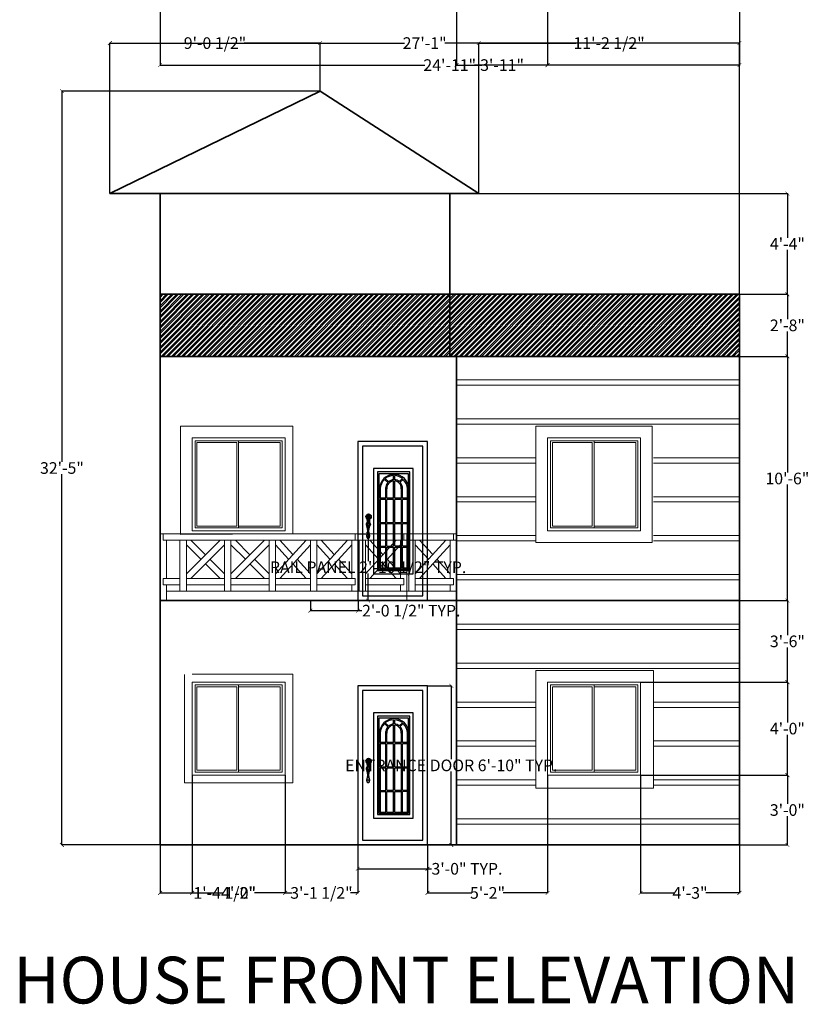
# Model space of a CAD drawing. Units: inches. Extents: x 528 to 2520, y -151 to 1354.
# Tile 28 of 41: x 2086 to 2493, y -151 to 357. Entities that reach past the tile are written whole.
import ezdxf

# ---------------------------------------------------------------- set-up
doc = ezdxf.new("R2010")
doc.units = ezdxf.units.IN
doc.header["$MEASUREMENT"] = 0
for name, color, linetype, lineweight in [('A-ANNO-DIMS', 2, 'Continuous', 18), ('A-ANNO-TEXT', 7, 'Continuous', 30), ('A-Door', 150, 'Continuous', 25), ('A-ELEV', 7, 'Continuous', 35), ('A-ELEV-FNSH', 7, 'Continuous', 18), ('A-ROOF', 7, 'Continuous', 35), ('KORKULUK', 4, 'Continuous', 20), ('WINDOWS', 2, 'Continuous', 20)]:
    doc.layers.add(name, color=color, linetype=linetype, lineweight=lineweight)
doc.layers.add('A-ELEV-PATT', color=175, linetype='Continuous', lineweight=13, true_color=0x4554a5)
doc.styles.get("Standard").update_dxf_attribs({"font": 'arial.ttf'})
doc.dimstyles.get("Standard").update_dxf_attribs({"dimtxt": 6, "dimasz": 2, "dimexe": 0.18, "dimexo": 0.0625, "dimgap": 0.09, "dimtad": 0, "dimtih": 1, "dimtoh": 1, "dimdec": 1, "dimzin": 0, "dimdsep": 46, "dimlunit": 3, "dimtxsty": 'Standard', "dimblk": 'ARCHTICK', "dimcen": 0.09, "dimadec": 0, "dimazin": 0, "dimtfac": 1, "dimtdec": 1, "dimtofl": 0, "dimtmove": 0, "dimatfit": 3, "dimfxl": 1, "dimtolj": 1, "dimtzin": 0, "dimarcsym": 0})

# ---------------------------------------------------------------- blocks, each defined once
blk = doc.blocks.new('*U29')
for p, q in [((1.5, 1.5), (1.5, 46.5)), ((1.5, 46.5), (24, 46.5)), ((24, 1.5), (24, 46.5)), ((24, 46.5), (46.5, 46.5)), ((46.5, 46.5), (46.5, 1.5)), ((24, 1.5), (1.5, 1.5)), ((46.5, 1.5), (24, 1.5))]:
    blk.add_line(p, q)
blk.add_lwpolyline([(0, 0), (0, 48), (48, 48), (48, 0)], close=True)
for points in [[(23, 45.5), (23, 2.5), (2.5, 2.5), (2.5, 45.5), (23, 45.5)], [(24, 45.5), (45.5, 45.5), (45.5, 2.5), (24, 2.5)]]:
    blk.add_lwpolyline(points)
blk = doc.blocks.new('DOOR-PANEL-ELEV-36')
for p, q in [((13.74, 62.55), (15.59, 60.9)), ((14.17, 62.94), (16, 61.3)), ((18.52, 62.33), (18.52, 64.55)), ((18.52, 52.78), (18.52, 61.75)), ((19.1, 62.33), (19.1, 64.53)), ((19.1, 52.78), (19.1, 61.75)), ((23.08, 62.95), (21.41, 61.45)), ((23.52, 62.56), (21.85, 61.06)), ((11.91, 57.81), (11.37, 57.81)), ((11.6, 57.81), (11.83, 57.81)), ((11.91, 57.81), (11.6, 57.81)), ((11.83, 57.81), (11.83, 58.12)), ((14.52, 52.78), (14.52, 58.42)), ((15.1, 52.78), (15.1, 58.42)), ((22.52, 52.78), (22.52, 58.12)), ((23.1, 52.78), (23.1, 58.12)), ((14.52, 52.78), (11.55, 52.78)), ((14.52, 52.2), (11.55, 52.2)), ((14.52, 40.31), (14.52, 52.2)), ((18.52, 52.78), (15.1, 52.78)), ((15.1, 40.31), (15.1, 52.2)), ((18.52, 52.2), (15.1, 52.2)), ((18.52, 40.33), (18.52, 52.2)), ((22.52, 52.78), (19.1, 52.78)), ((19.1, 40.33), (19.1, 52.2)), ((22.52, 52.2), (19.1, 52.2)), ((22.52, 40.35), (22.52, 52.2)), ((25.61, 52.78), (23.1, 52.78)), ((25.61, 52.2), (23.1, 52.2)), ((23.1, 40.36), (23.1, 52.2)), ((5.17, 42.07), (5.17, 40.37)), ((5.85, 42.01), (5.85, 40.4)), ((5.17, 38.33), (5.17, 34.66)), ((5.6, 38.27), (5.6, 34.75)), ((11.55, 40.29), (14.52, 40.31)), ((11.55, 39.71), (14.52, 39.73)), ((14.52, 28.17), (14.52, 39.73)), ((15.1, 40.31), (18.52, 40.33)), ((15.1, 39.73), (18.52, 39.75)), ((15.1, 28.17), (15.1, 39.73)), ((18.52, 28.19), (18.52, 39.75)), ((19.1, 40.33), (22.52, 40.35)), ((19.1, 39.76), (22.52, 39.78)), ((19.1, 28.19), (19.1, 39.76)), ((22.52, 16.87), (22.52, 39.78)), ((23.1, 40.36), (25.61, 40.37)), ((23.1, 39.78), (25.61, 39.8)), ((23.1, 28.22), (23.1, 39.78)), ((10.97, 16.3), (10.97, 27.86)), ((11.55, 28.15), (14.52, 28.17)), ((11.55, 27.57), (14.52, 27.59)), ((14.52, 16.87), (14.52, 27.59)), ((15.1, 28.17), (18.52, 28.19)), ((15.1, 27.59), (18.52, 27.61)), ((15.1, 16.87), (15.1, 27.59)), ((18.52, 16.87), (18.52, 27.61)), ((19.1, 28.19), (22.52, 28.21)), ((19.1, 27.62), (22.52, 27.64)), ((19.1, 16.87), (19.1, 27.62)), ((23.1, 28.22), (25.61, 28.23)), ((23.1, 27.64), (25.61, 27.66)), ((23.1, 16.87), (23.1, 27.64)), ((26.23, 16.3), (22.52, 16.3))]:
    blk.add_line(p, q)
for points in [[(36, 0), (36, 82.04), (0, 82.04), (0, 0)], [(33.55, 2.45), (33.55, 79.6), (2.45, 79.6), (2.45, 2.45)], [(28.61, 13.88), (28.61, 68.17), (8.2, 68.17), (8.2, 13.88)], [(26.88, 15.61), (26.88, 66.44), (10.28, 66.44), (10.28, 15.61)], [(26.19, 16.3), (26.19, 65.4), (10.97, 65.4), (10.97, 16.3)], [(6.31, 42.2), (6.31, 44.42), (4.84, 44.42), (4.84, 42.2)], [(5.86, 42.6), (5.86, 43.89), (5.29, 43.89), (5.29, 42.6)], [(6, 38.52), (6, 40.2), (4.97, 40.2), (4.97, 38.52)]]:
    blk.add_lwpolyline(points, close=True)
for points in [[(11.55, 58.12), (11.55, 52.78)], [(25.61, 52.78), (25.61, 59.08)], [(11.55, 52.2), (11.55, 40.29)], [(25.61, 40.37), (25.61, 52.2)], [(11.55, 39.71), (11.55, 16.87), (14.52, 16.87)], [(25.61, 16.87), (25.61, 39.8)], [(15.1, 16.87), (18.52, 16.87)], [(19.1, 16.87), (22.52, 16.87)], [(23.1, 16.87), (25.61, 16.87)]]:
    blk.add_lwpolyline(points)
blk.add_lwpolyline([(6.03, 33.36, -0.045721), (5.98, 32.78, -0.059301), (5.85, 32.36, -0.101058), (5.61, 32.02, -0.189275), (5.4, 31.94, -0.189275), (5.19, 32.02, -0.101058), (4.95, 32.36, -0.059301), (4.82, 32.78, -0.045721), (4.77, 33.36, -0.045721), (4.82, 33.94, -0.059301), (4.95, 34.37, -0.101058), (5.19, 34.7, -0.189275), (5.4, 34.78, -0.189275), (5.61, 34.7, -0.101058), (5.85, 34.37, -0.059301), (5.98, 33.94, -0.045721)], format="xyb", close=True)
for centre, radius in [((5.61, 43.34), 1.35), ((5.61, 43.34), 0.752), ((5.61, 43.34), 0.392), ((5.5, 39.36), 1.05), ((5.5, 39.36), 0.55), ((5.39, 33.33), 0.278)]:
    blk.add_circle(centre, radius)
for centre, radius, start, end in [((18.79, 57.56), 7.57, 1.2104, 178.7896), ((18.64, 57.56), 6.99, 134.4827, 178.7896), ((18.64, 57.56), 6.99, 90.9488, 129.7225), ((18.79, 58.05), 3.71, 94.2253, 185.0935), ((18.79, 58.05), 4.29, 93.6561, 130.6705), ((19.88, 38.4), 27.02, 89.5366, 91.7216), ((18.64, 57.56), 6.99, 50.4895, 86.2145), ((18.79, 58.05), 4.29, 52.4124, 85.9434), ((18.79, 58.05), 3.71, 354.9065, 85.3116), ((18.79, 58.05), 4.29, 354.9065, 44.6486), ((18.64, 57.56), 6.99, 1.2104, 45.7292), ((18.79, 58.05), 4.29, 138.3994, 185.0935), ((2.68, 41.16), 2.34, 319.4574, 32.1732), ((8.36, 40.89), 2.34, 142.3675, 215.0833), ((-1.32, 36.06), 6.5, 338.0978, 21.9022), ((12.13, 36.06), 6.5, 158.0978, 201.9022)]:
    blk.add_arc(centre, radius, start, end)
blk = doc.blocks.new('BALCONY-RAIL-PANEL')
for p, q in [((0, 31.17), (0, 4.92)), ((3.28, 31.17), (3.28, 4.92)), ((3.28, 13.91), (19.11, 31.17)), ((5.51, 31.17), (12.31, 23.75)), ((21.34, 31.17), (21.34, 11.48)), ((24.62, 34.45), (24.62, 0)), ((3.28, 28.74), (10.08, 21.33)), ((5.51, 11.48), (21.34, 28.74)), ((14.54, 21.33), (21.34, 13.91)), ((12.31, 18.9), (19.11, 11.48)), ((3.28, 11.48), (23.05, 11.48)), ((3.28, 8.2), (23.05, 8.2)), ((21.34, 8.2), (21.34, 4.92))]:
    blk.add_line(p, q)
for points in [[(23.05, 31.17), (23.05, 34.45)], [(23.05, 8.2), (23.05, 11.48)]]:
    blk.add_lwpolyline(points)
blk = doc.blocks.new('_ArchTick')
at = {"color": 0, "linetype": 'ByBlock', "const_width": 0.15}
blk.add_lwpolyline([(-0.5, -0.5), (0.5, 0.5)], dxfattribs=at)
blk = doc.blocks.new('*D88')
at = {"layer": 'A-ANNO-DIMS', "color": 0, "lineweight": -2, "transparency": 16777216}
for p, q in [((2260.28, 91.5), (2265.56, 91.5)), ((2265.38, 91.5), (2265.38, 77.47)), ((2265.38, 57.05), (2265.38, 71.08)), ((2260.28, 57.05), (2265.56, 57.05))]:
    blk.add_line(p, q, dxfattribs=at)
at = {"layer": 'Defpoints', "color": 0, "transparency": 16777216}
for p in [(2260.22, 91.5), (2265.38, 91.5), (2260.22, 57.05)]:
    blk.add_point(p, dxfattribs=at)
at = {"layer": 'A-ANNO-DIMS', "color": 0, "lineweight": -2, "transparency": 16777216, "xscale": 2, "yscale": 2, "zscale": 2}
for p, rotation in [((2265.38, 91.5), 90), ((2265.38, 57.05), 270)]:
    blk.add_blockref('_ArchTick', p, dxfattribs=dict(at, rotation=rotation))
at = {"layer": 'A-ANNO-DIMS', "color": 0, "transparency": 16777216, "insert": (2265.38, 74.27), "char_height": 6, "attachment_point": 5}
blk.add_mtext('\\A1;RAIL PANEL 2\'-10 1/2" TYP.', dxfattribs=at)
blk = doc.blocks.new('*D89')
at = {"layer": 'A-ANNO-DIMS', "color": 0, "lineweight": -2, "transparency": 16777216}
for p, q in [((2235.6, 56.99), (2235.6, 51.7)), ((2260.22, 56.99), (2260.22, 51.7)), ((2235.6, 51.88), (2260.22, 51.88)), ((2260.22, 51.88), (2262.22, 51.88))]:
    blk.add_line(p, q, dxfattribs=at)
at = {"layer": 'Defpoints', "color": 0, "transparency": 16777216}
for p in [(2235.6, 57.05), (2260.22, 57.05), (2260.22, 51.88)]:
    blk.add_point(p, dxfattribs=at)
at = {"layer": 'A-ANNO-DIMS', "color": 0, "lineweight": -2, "transparency": 16777216, "xscale": 2, "yscale": 2, "zscale": 2, "rotation": 180}
blk.add_blockref('_ArchTick', (2235.6, 51.88), dxfattribs=at)
at = {"layer": 'A-ANNO-DIMS', "color": 0, "lineweight": -2, "transparency": 16777216, "xscale": 2, "yscale": 2, "zscale": 2}
blk.add_blockref('_ArchTick', (2260.22, 51.88), dxfattribs=at)
at = {"layer": 'A-ANNO-DIMS', "color": 0, "transparency": 16777216, "insert": (2287.64, 51.88), "char_height": 6, "attachment_point": 5}
blk.add_mtext('\\A1;2\'-0 1/2" TYP.', dxfattribs=at)
blk = doc.blocks.new('*D90')
at = {"layer": 'A-ANNO-DIMS', "color": 0, "lineweight": -2, "transparency": 16777216}
for p, q in [((2296.08, 13.09), (2308.5, 13.09)), ((2308.32, 13.09), (2308.32, -24.73)), ((2308.32, -68.95), (2308.32, -31.12)), ((2296.08, -68.95), (2308.5, -68.95))]:
    blk.add_line(p, q, dxfattribs=at)
at = {"layer": 'Defpoints', "color": 0, "transparency": 16777216}
for p in [(2296.02, 13.09), (2308.32, 13.09), (2296.02, -68.95)]:
    blk.add_point(p, dxfattribs=at)
at = {"layer": 'A-ANNO-DIMS', "color": 0, "lineweight": -2, "transparency": 16777216, "xscale": 2, "yscale": 2, "zscale": 2}
for p, rotation in [((2308.32, 13.09), 90), ((2308.32, -68.95), 270)]:
    blk.add_blockref('_ArchTick', p, dxfattribs=dict(at, rotation=rotation))
at = {"layer": 'A-ANNO-DIMS', "color": 0, "transparency": 16777216, "insert": (2308.32, -27.93), "char_height": 6, "attachment_point": 5}
blk.add_mtext('\\A1;ENTRANCE DOOR 6\'-10" TYP.', dxfattribs=at)
blk = doc.blocks.new('*D91')
at = {"layer": 'A-ANNO-DIMS', "color": 0, "lineweight": -2, "transparency": 16777216}
for p, q in [((2260.02, -69.01), (2260.02, -81.44)), ((2296.02, -69.01), (2296.02, -81.44)), ((2260.02, -81.26), (2296.02, -81.26)), ((2296.02, -81.26), (2298.02, -81.26))]:
    blk.add_line(p, q, dxfattribs=at)
at = {"layer": 'Defpoints', "color": 0, "transparency": 16777216}
for p in [(2260.02, -68.95), (2296.02, -68.95), (2296.02, -81.26)]:
    blk.add_point(p, dxfattribs=at)
at = {"layer": 'A-ANNO-DIMS', "color": 0, "lineweight": -2, "transparency": 16777216, "xscale": 2, "yscale": 2, "zscale": 2, "rotation": 180}
blk.add_blockref('_ArchTick', (2260.02, -81.26), dxfattribs=at)
at = {"layer": 'A-ANNO-DIMS', "color": 0, "lineweight": -2, "transparency": 16777216, "xscale": 2, "yscale": 2, "zscale": 2}
blk.add_blockref('_ArchTick', (2296.02, -81.26), dxfattribs=at)
at = {"layer": 'A-ANNO-DIMS', "color": 0, "transparency": 16777216, "insert": (2316.39, -81.26), "char_height": 6, "attachment_point": 5}
blk.add_mtext('\\A1;3\'-0" TYP.', dxfattribs=at)
blk = doc.blocks.new('*D94')
at = {"layer": 'A-ANNO-DIMS', "color": 0, "lineweight": -2, "transparency": 16777216}
for p, q in [((2158.01, 360.88), (2158.01, 333.11)), ((2457.01, 360.88), (2457.01, 333.11)), ((2158.01, 333.29), (2294.73, 333.29)), ((2457.01, 333.29), (2320.29, 333.29))]:
    blk.add_line(p, q, dxfattribs=at)
at = {"layer": 'Defpoints', "color": 0, "transparency": 16777216}
for p in [(2158.01, 360.94), (2457.01, 360.94), (2457.01, 333.29)]:
    blk.add_point(p, dxfattribs=at)
at = {"layer": 'A-ANNO-DIMS', "color": 0, "lineweight": -2, "transparency": 16777216, "xscale": 2, "yscale": 2, "zscale": 2, "rotation": 180}
blk.add_blockref('_ArchTick', (2158.01, 333.29), dxfattribs=at)
at = {"layer": 'A-ANNO-DIMS', "color": 0, "lineweight": -2, "transparency": 16777216, "xscale": 2, "yscale": 2, "zscale": 2}
blk.add_blockref('_ArchTick', (2457.01, 333.29), dxfattribs=at)
at = {"layer": 'A-ANNO-DIMS', "color": 0, "transparency": 16777216, "insert": (2307.51, 333.29), "char_height": 6, "attachment_point": 5}
blk.add_mtext('\\A1;24\'-11"', dxfattribs=at)
blk = doc.blocks.new('*D100')
at = {"layer": 'A-ANNO-DIMS', "color": 0, "lineweight": -2, "transparency": 16777216}
for p, q in [((2311.01, 396.88), (2311.01, 333.11)), ((2358.01, 396.88), (2358.01, 333.11)), ((2311.01, 333.29), (2324.12, 333.29)), ((2358.01, 333.29), (2344.91, 333.29))]:
    blk.add_line(p, q, dxfattribs=at)
at = {"layer": 'Defpoints', "color": 0, "transparency": 16777216}
for p in [(2311.01, 396.94), (2358.01, 396.94), (2358.01, 333.29)]:
    blk.add_point(p, dxfattribs=at)
at = {"layer": 'A-ANNO-DIMS', "color": 0, "lineweight": -2, "transparency": 16777216, "xscale": 2, "yscale": 2, "zscale": 2, "rotation": 180}
blk.add_blockref('_ArchTick', (2311.01, 333.29), dxfattribs=at)
at = {"layer": 'A-ANNO-DIMS', "color": 0, "lineweight": -2, "transparency": 16777216, "xscale": 2, "yscale": 2, "zscale": 2}
blk.add_blockref('_ArchTick', (2358.01, 333.29), dxfattribs=at)
at = {"layer": 'A-ANNO-DIMS', "color": 0, "transparency": 16777216, "insert": (2334.51, 333.29), "char_height": 6, "attachment_point": 5}
blk.add_mtext('\\A1;3\'-11"', dxfattribs=at)
blk = doc.blocks.new('*D101')
at = {"layer": 'A-ANNO-DIMS', "color": 0, "lineweight": -2, "transparency": 16777216}
for p, q in [((2132.13, 267.11), (2132.13, 344.81)), ((2132.13, 344.63), (2284.13, 344.63)), ((2457.01, 344.63), (2305.02, 344.63)), ((2457.01, 215.11), (2457.01, 344.81))]:
    blk.add_line(p, q, dxfattribs=at)
at = {"layer": 'Defpoints', "color": 0, "transparency": 16777216}
for p in [(2457.01, 344.63), (2132.13, 267.05), (2457.01, 215.05)]:
    blk.add_point(p, dxfattribs=at)
at = {"layer": 'A-ANNO-DIMS', "color": 0, "lineweight": -2, "transparency": 16777216, "xscale": 2, "yscale": 2, "zscale": 2, "rotation": 180}
blk.add_blockref('_ArchTick', (2132.13, 344.63), dxfattribs=at)
at = {"layer": 'A-ANNO-DIMS', "color": 0, "lineweight": -2, "transparency": 16777216, "xscale": 2, "yscale": 2, "zscale": 2}
blk.add_blockref('_ArchTick', (2457.01, 344.63), dxfattribs=at)
at = {"layer": 'A-ANNO-DIMS', "color": 0, "transparency": 16777216, "insert": (2294.57, 344.63), "char_height": 6, "attachment_point": 5}
blk.add_mtext('\\A1;27\'-1"', dxfattribs=at)
blk = doc.blocks.new('*D102')
at = {"layer": 'A-ANNO-DIMS', "color": 0, "lineweight": -2, "transparency": 16777216}
for p, q in [((2240.53, 319.88), (2107.2, 319.88)), ((2107.38, 319.88), (2107.38, 128.62)), ((2107.38, -68.95), (2107.38, 122.31)), ((2157.95, -68.95), (2107.2, -68.95))]:
    blk.add_line(p, q, dxfattribs=at)
at = {"layer": 'Defpoints', "color": 0, "transparency": 16777216}
for p in [(2240.59, 319.88), (2107.38, -68.95), (2158.01, -68.95)]:
    blk.add_point(p, dxfattribs=at)
at = {"layer": 'A-ANNO-DIMS', "color": 0, "lineweight": -2, "transparency": 16777216, "xscale": 2, "yscale": 2, "zscale": 2}
for p, rotation in [((2107.38, 319.88), 90), ((2107.38, -68.95), 270)]:
    blk.add_blockref('_ArchTick', p, dxfattribs=dict(at, rotation=rotation))
at = {"layer": 'A-ANNO-DIMS', "color": 0, "transparency": 16777216, "insert": (2107.38, 125.46), "char_height": 6, "attachment_point": 5}
blk.add_mtext('\\A1;32\'-5"', dxfattribs=at)
blk = doc.blocks.new('*D103')
at = {"layer": 'A-ANNO-DIMS', "color": 0, "lineweight": -2, "transparency": 16777216}
for p, q in [((2457.07, 183.05), (2481.94, 183.05)), ((2481.76, 183.05), (2481.76, 123.2)), ((2481.76, 57.05), (2481.76, 116.9)), ((2457.07, 57.05), (2481.94, 57.05))]:
    blk.add_line(p, q, dxfattribs=at)
at = {"layer": 'Defpoints', "color": 0, "transparency": 16777216}
for p in [(2457.01, 183.05), (2481.76, 183.05), (2457.01, 57.05)]:
    blk.add_point(p, dxfattribs=at)
at = {"layer": 'A-ANNO-DIMS', "color": 0, "lineweight": -2, "transparency": 16777216, "xscale": 2, "yscale": 2, "zscale": 2}
for p, rotation in [((2481.76, 183.05), 90), ((2481.76, 57.05), 270)]:
    blk.add_blockref('_ArchTick', p, dxfattribs=dict(at, rotation=rotation))
at = {"layer": 'A-ANNO-DIMS', "color": 0, "transparency": 16777216, "insert": (2481.76, 120.05), "char_height": 6, "attachment_point": 5}
blk.add_mtext('\\A1;10\'-6"', dxfattribs=at)
blk = doc.blocks.new('*D104')
at = {"layer": 'A-ANNO-DIMS', "color": 0, "lineweight": -2, "transparency": 16777216}
for p, q in [((2457.07, 215.05), (2481.94, 215.05)), ((2481.76, 215.05), (2481.76, 202.2)), ((2481.76, 183.05), (2481.76, 195.9)), ((2457.07, 183.05), (2481.94, 183.05))]:
    blk.add_line(p, q, dxfattribs=at)
at = {"layer": 'Defpoints', "color": 0, "transparency": 16777216}
for p in [(2457.01, 215.05), (2481.76, 215.05), (2457.01, 183.05)]:
    blk.add_point(p, dxfattribs=at)
at = {"layer": 'A-ANNO-DIMS', "color": 0, "lineweight": -2, "transparency": 16777216, "xscale": 2, "yscale": 2, "zscale": 2}
for p, rotation in [((2481.76, 215.05), 90), ((2481.76, 183.05), 270)]:
    blk.add_blockref('_ArchTick', p, dxfattribs=dict(at, rotation=rotation))
at = {"layer": 'A-ANNO-DIMS', "color": 0, "transparency": 16777216, "insert": (2481.76, 199.05), "char_height": 6, "attachment_point": 5}
blk.add_mtext('\\A1;2\'-8"', dxfattribs=at)
blk = doc.blocks.new('*D105')
at = {"layer": 'A-ANNO-DIMS', "color": 0, "lineweight": -2, "transparency": 16777216}
for p, q in [((2322.553492, 267.050466), (2481.942076, 267.050466)), ((2481.762076, 267.050466), (2481.762076, 244.140466)), ((2481.762076, 215.050466), (2481.762076, 237.960466)), ((2457.074576, 215.050466), (2481.942076, 215.050466))]:
    blk.add_line(p, q, dxfattribs=at)
at = {"layer": 'Defpoints', "color": 0, "transparency": 16777216}
for p in [(2322.490992, 267.050466), (2481.762076, 267.050466), (2457.012076, 215.050466)]:
    blk.add_point(p, dxfattribs=at)
at = {"layer": 'A-ANNO-DIMS', "color": 0, "lineweight": -2, "transparency": 16777216, "xscale": 2, "yscale": 2, "zscale": 2}
for p, rotation in [((2481.762076, 267.050466), 90), ((2481.762076, 215.050466), 270)]:
    blk.add_blockref('_ArchTick', p, dxfattribs=dict(at, rotation=rotation))
at = {"layer": 'A-ANNO-DIMS', "color": 0, "transparency": 16777216, "insert": (2481.762076, 241.050466), "char_height": 6, "attachment_point": 5}
blk.add_mtext('\\A1;4\'-4"', dxfattribs=at)
blk = doc.blocks.new('*D106')
at = {"layer": 'A-ANNO-DIMS', "color": 0, "lineweight": -2, "transparency": 16777216}
for p, q in [((2322.49, 267.11), (2322.49, 344.81)), ((2322.49, 344.63), (2372.65, 344.63)), ((2457.01, 344.63), (2406.86, 344.63)), ((2457.01, 215.11), (2457.01, 344.81))]:
    blk.add_line(p, q, dxfattribs=at)
at = {"layer": 'Defpoints', "color": 0, "transparency": 16777216}
for p in [(2457.01, 344.63), (2322.49, 267.05), (2457.01, 215.05)]:
    blk.add_point(p, dxfattribs=at)
at = {"layer": 'A-ANNO-DIMS', "color": 0, "lineweight": -2, "transparency": 16777216, "xscale": 2, "yscale": 2, "zscale": 2, "rotation": 180}
blk.add_blockref('_ArchTick', (2322.49, 344.63), dxfattribs=at)
at = {"layer": 'A-ANNO-DIMS', "color": 0, "lineweight": -2, "transparency": 16777216, "xscale": 2, "yscale": 2, "zscale": 2}
blk.add_blockref('_ArchTick', (2457.01, 344.63), dxfattribs=at)
at = {"layer": 'A-ANNO-DIMS', "color": 0, "transparency": 16777216, "insert": (2389.75, 344.63), "char_height": 6, "attachment_point": 5}
blk.add_mtext('\\A1;11\'-2 1/2"', dxfattribs=at)
blk = doc.blocks.new('*D107')
at = {"layer": 'A-ANNO-DIMS', "color": 0, "lineweight": -2, "transparency": 16777216}
for p, q in [((2132.13, 267.11), (2132.13, 344.81)), ((2132.13, 344.63), (2171.31, 344.63)), ((2240.59, 344.63), (2201.42, 344.63)), ((2240.59, 319.94), (2240.59, 344.81))]:
    blk.add_line(p, q, dxfattribs=at)
at = {"layer": 'Defpoints', "color": 0, "transparency": 16777216}
for p in [(2240.59, 344.63), (2240.59, 319.88), (2132.13, 267.05)]:
    blk.add_point(p, dxfattribs=at)
at = {"layer": 'A-ANNO-DIMS', "color": 0, "lineweight": -2, "transparency": 16777216, "xscale": 2, "yscale": 2, "zscale": 2, "rotation": 180}
blk.add_blockref('_ArchTick', (2132.13, 344.63), dxfattribs=at)
at = {"layer": 'A-ANNO-DIMS', "color": 0, "lineweight": -2, "transparency": 16777216, "xscale": 2, "yscale": 2, "zscale": 2}
blk.add_blockref('_ArchTick', (2240.59, 344.63), dxfattribs=at)
at = {"layer": 'A-ANNO-DIMS', "color": 0, "transparency": 16777216, "insert": (2186.36, 344.63), "char_height": 6, "attachment_point": 5}
blk.add_mtext('\\A1;9\'-0 1/2"', dxfattribs=at)
blk = doc.blocks.new('*D108')
at = {"layer": 'A-ANNO-DIMS', "color": 0, "lineweight": -2, "transparency": 16777216}
for p, q in [((2174.56, -33.01), (2174.56, -93.88)), ((2222.56, -33.01), (2222.56, -93.88)), ((2174.56, -93.7), (2190.37, -93.7)), ((2222.56, -93.7), (2206.74, -93.7))]:
    blk.add_line(p, q, dxfattribs=at)
at = {"layer": 'Defpoints', "color": 0, "transparency": 16777216}
for p in [(2174.56, -32.95), (2222.56, -32.95), (2222.56, -93.7)]:
    blk.add_point(p, dxfattribs=at)
at = {"layer": 'A-ANNO-DIMS', "color": 0, "lineweight": -2, "transparency": 16777216, "xscale": 2, "yscale": 2, "zscale": 2, "rotation": 180}
blk.add_blockref('_ArchTick', (2174.56, -93.7), dxfattribs=at)
at = {"layer": 'A-ANNO-DIMS', "color": 0, "lineweight": -2, "transparency": 16777216, "xscale": 2, "yscale": 2, "zscale": 2}
blk.add_blockref('_ArchTick', (2222.56, -93.7), dxfattribs=at)
at = {"layer": 'A-ANNO-DIMS', "color": 0, "transparency": 16777216, "insert": (2198.56, -93.7), "char_height": 6, "attachment_point": 5}
blk.add_mtext('\\A1;4\'-0"', dxfattribs=at)
blk = doc.blocks.new('*D109')
at = {"layer": 'A-ANNO-DIMS', "color": 0, "lineweight": -2, "transparency": 16777216}
for p, q in [((2406.07, 15.05), (2481.94, 15.05)), ((2481.76, 15.05), (2481.76, -5.8)), ((2481.76, -32.95), (2481.76, -12.1)), ((2406.07, -32.95), (2481.94, -32.95))]:
    blk.add_line(p, q, dxfattribs=at)
at = {"layer": 'Defpoints', "color": 0, "transparency": 16777216}
for p in [(2406.01, 15.05), (2481.76, 15.05), (2406.01, -32.95)]:
    blk.add_point(p, dxfattribs=at)
at = {"layer": 'A-ANNO-DIMS', "color": 0, "lineweight": -2, "transparency": 16777216, "xscale": 2, "yscale": 2, "zscale": 2}
for p, rotation in [((2481.76, 15.05), 90), ((2481.76, -32.95), 270)]:
    blk.add_blockref('_ArchTick', p, dxfattribs=dict(at, rotation=rotation))
at = {"layer": 'A-ANNO-DIMS', "color": 0, "transparency": 16777216, "insert": (2481.76, -8.95), "char_height": 6, "attachment_point": 5}
blk.add_mtext('\\A1;4\'-0"', dxfattribs=at)
blk = doc.blocks.new('*D110')
at = {"layer": 'A-ANNO-DIMS', "color": 0, "lineweight": -2, "transparency": 16777216}
for p, q in [((2174.56, -33.01), (2174.56, -93.88)), ((2158.01, -69.01), (2158.01, -93.88)), ((2158.01, -93.7), (2174.56, -93.7)), ((2174.56, -93.7), (2176.56, -93.7))]:
    blk.add_line(p, q, dxfattribs=at)
at = {"layer": 'Defpoints', "color": 0, "transparency": 16777216}
for p in [(2174.56, -32.95), (2158.01, -68.95), (2174.56, -93.7)]:
    blk.add_point(p, dxfattribs=at)
at = {"layer": 'A-ANNO-DIMS', "color": 0, "lineweight": -2, "transparency": 16777216, "xscale": 2, "yscale": 2, "zscale": 2, "rotation": 180}
blk.add_blockref('_ArchTick', (2158.01, -93.7), dxfattribs=at)
at = {"layer": 'A-ANNO-DIMS', "color": 0, "lineweight": -2, "transparency": 16777216, "xscale": 2, "yscale": 2, "zscale": 2}
blk.add_blockref('_ArchTick', (2174.56, -93.7), dxfattribs=at)
at = {"layer": 'A-ANNO-DIMS', "color": 0, "transparency": 16777216, "insert": (2191.33, -93.7), "char_height": 6, "attachment_point": 5}
blk.add_mtext('\\A1;1\'-4 1/2"', dxfattribs=at)
blk = doc.blocks.new('*D111')
at = {"layer": 'A-ANNO-DIMS', "color": 0, "lineweight": -2, "transparency": 16777216}
for p, q in [((2222.56, -33.01), (2222.56, -93.88)), ((2260.02, -69.01), (2260.02, -93.88)), ((2222.56, -93.7), (2226.23, -93.7)), ((2260.02, -93.7), (2256.34, -93.7))]:
    blk.add_line(p, q, dxfattribs=at)
at = {"layer": 'Defpoints', "color": 0, "transparency": 16777216}
for p in [(2222.56, -32.95), (2260.02, -68.95), (2260.02, -93.7)]:
    blk.add_point(p, dxfattribs=at)
at = {"layer": 'A-ANNO-DIMS', "color": 0, "lineweight": -2, "transparency": 16777216, "xscale": 2, "yscale": 2, "zscale": 2, "rotation": 180}
blk.add_blockref('_ArchTick', (2222.56, -93.7), dxfattribs=at)
at = {"layer": 'A-ANNO-DIMS', "color": 0, "lineweight": -2, "transparency": 16777216, "xscale": 2, "yscale": 2, "zscale": 2}
blk.add_blockref('_ArchTick', (2260.02, -93.7), dxfattribs=at)
at = {"layer": 'A-ANNO-DIMS', "color": 0, "transparency": 16777216, "insert": (2241.29, -93.7), "char_height": 6, "attachment_point": 5}
blk.add_mtext('\\A1;3\'-1 1/2"', dxfattribs=at)
blk = doc.blocks.new('*D112')
at = {"layer": 'A-ANNO-DIMS', "color": 0, "lineweight": -2, "transparency": 16777216}
for p, q in [((2358.01, -33.01), (2358.01, -93.88)), ((2296.02, -69.01), (2296.02, -93.88)), ((2296.02, -93.7), (2318.95, -93.7)), ((2358.01, -93.7), (2335.08, -93.7))]:
    blk.add_line(p, q, dxfattribs=at)
at = {"layer": 'Defpoints', "color": 0, "transparency": 16777216}
for p in [(2358.01, -32.95), (2296.02, -68.95), (2358.01, -93.7)]:
    blk.add_point(p, dxfattribs=at)
at = {"layer": 'A-ANNO-DIMS', "color": 0, "lineweight": -2, "transparency": 16777216, "xscale": 2, "yscale": 2, "zscale": 2, "rotation": 180}
blk.add_blockref('_ArchTick', (2296.02, -93.7), dxfattribs=at)
at = {"layer": 'A-ANNO-DIMS', "color": 0, "lineweight": -2, "transparency": 16777216, "xscale": 2, "yscale": 2, "zscale": 2}
blk.add_blockref('_ArchTick', (2358.01, -93.7), dxfattribs=at)
at = {"layer": 'A-ANNO-DIMS', "color": 0, "transparency": 16777216, "insert": (2327.01, -93.7), "char_height": 6, "attachment_point": 5}
blk.add_mtext('\\A1;5\'-2"', dxfattribs=at)
blk = doc.blocks.new('*D113')
at = {"layer": 'A-ANNO-DIMS', "color": 0, "lineweight": -2, "transparency": 16777216}
for p, q in [((2406.07, -32.95), (2481.94, -32.95)), ((2481.76, -32.95), (2481.76, -47.79)), ((2481.76, -68.95), (2481.76, -54.11)), ((2457.07, -68.95), (2481.94, -68.95))]:
    blk.add_line(p, q, dxfattribs=at)
at = {"layer": 'Defpoints', "color": 0, "transparency": 16777216}
for p in [(2406.01, -32.95), (2481.76, -32.95), (2457.01, -68.95)]:
    blk.add_point(p, dxfattribs=at)
at = {"layer": 'A-ANNO-DIMS', "color": 0, "lineweight": -2, "transparency": 16777216, "xscale": 2, "yscale": 2, "zscale": 2}
for p, rotation in [((2481.76, -32.95), 90), ((2481.76, -68.95), 270)]:
    blk.add_blockref('_ArchTick', p, dxfattribs=dict(at, rotation=rotation))
at = {"layer": 'A-ANNO-DIMS', "color": 0, "transparency": 16777216, "insert": (2481.76, -50.95), "char_height": 6, "attachment_point": 5}
blk.add_mtext('\\A1;3\'-0"', dxfattribs=at)
blk = doc.blocks.new('*D114')
at = {"layer": 'A-ANNO-DIMS', "color": 0, "lineweight": -2, "transparency": 16777216}
for p, q in [((2457.07, 57.05), (2481.94, 57.05)), ((2481.76, 57.05), (2481.76, 39.21)), ((2481.76, 15.05), (2481.76, 32.89)), ((2406.07, 15.05), (2481.94, 15.05))]:
    blk.add_line(p, q, dxfattribs=at)
at = {"layer": 'Defpoints', "color": 0, "transparency": 16777216}
for p in [(2457.01, 57.05), (2481.76, 57.05), (2406.01, 15.05)]:
    blk.add_point(p, dxfattribs=at)
at = {"layer": 'A-ANNO-DIMS', "color": 0, "lineweight": -2, "transparency": 16777216, "xscale": 2, "yscale": 2, "zscale": 2}
for p, rotation in [((2481.76, 57.05), 90), ((2481.76, 15.05), 270)]:
    blk.add_blockref('_ArchTick', p, dxfattribs=dict(at, rotation=rotation))
at = {"layer": 'A-ANNO-DIMS', "color": 0, "transparency": 16777216, "insert": (2481.76, 36.05), "char_height": 6, "attachment_point": 5}
blk.add_mtext('\\A1;3\'-6"', dxfattribs=at)
blk = doc.blocks.new('*D115')
at = {"layer": 'A-ANNO-DIMS', "color": 0, "lineweight": -2, "transparency": 16777216}
for p, q in [((2406.01, -33.01), (2406.01, -93.88)), ((2457.01, -69.01), (2457.01, -93.88)), ((2406.01, -93.7), (2423.33, -93.7)), ((2457.01, -93.7), (2439.7, -93.7))]:
    blk.add_line(p, q, dxfattribs=at)
at = {"layer": 'Defpoints', "color": 0, "transparency": 16777216}
for p in [(2406.01, -32.95), (2457.01, -68.95), (2457.01, -93.7)]:
    blk.add_point(p, dxfattribs=at)
at = {"layer": 'A-ANNO-DIMS', "color": 0, "lineweight": -2, "transparency": 16777216, "xscale": 2, "yscale": 2, "zscale": 2, "rotation": 180}
blk.add_blockref('_ArchTick', (2406.01, -93.7), dxfattribs=at)
at = {"layer": 'A-ANNO-DIMS', "color": 0, "lineweight": -2, "transparency": 16777216, "xscale": 2, "yscale": 2, "zscale": 2}
blk.add_blockref('_ArchTick', (2457.01, -93.7), dxfattribs=at)
at = {"layer": 'A-ANNO-DIMS', "color": 0, "transparency": 16777216, "insert": (2431.51, -93.7), "char_height": 6, "attachment_point": 5}
blk.add_mtext('\\A1;4\'-3"', dxfattribs=at)

msp = doc.modelspace()

# ---------------------------------------------------------------- hatches: boundary and pattern name
at = {"layer": 'A-ELEV-PATT'}
h = msp.add_hatch(dxfattribs=at)
h.set_pattern_fill('ANSI32', color=256, scale=5)
h.paths.add_polyline_path([(2457.01, 215.05), (2307.51, 215.05), (2307.51, 183.05), (2457.01, 183.05)])
h.paths.add_polyline_path([(2307.51, 215.05), (2158.01, 215.05), (2158.01, 183.05), (2307.51, 183.05)])

# ---------------------------------------------------------------- linework, layer by layer
at = {"layer": 'A-ELEV'}
for p, q in [((2158.01, 183.05), (2158.01, 267.05)), ((2307.51, 183.05), (2307.51, 267.05)), ((2457.01, 215.05), (2158.01, 215.05)), ((2158.01, 215.05), (2158.01, 183.05)), ((2457.01, 183.05), (2457.01, 215.05)), ((2158.01, 57.05), (2158.01, 183.05)), ((2158.01, 183.05), (2457.01, 183.05)), ((2311.01, 51.05), (2311.01, 183.05)), ((2457.01, 57.05), (2457.01, 183.05)), ((2158.01, -68.95), (2158.01, 57.05)), ((2158.01, 57.05), (2457.01, 57.05)), ((2158.01, 57.05), (2457.01, 57.05)), ((2457.01, -68.95), (2457.01, 57.05)), ((2311.01, -68.95), (2311.01, 51.05)), ((2158.01, -68.95), (2457.01, -68.95))]:
    msp.add_line(p, q, dxfattribs=at)
at = {"layer": 'A-ELEV-FNSH'}
for points in [[(2311.01, 170.86), (2457.01, 170.86), (2457.01, 168.14), (2311.01, 168.14)], [(2311.01, 150.79), (2457.01, 150.79), (2457.01, 148.08), (2311.01, 148.08)], [(2311.01, 70.52), (2457.01, 70.52), (2457.01, 67.8), (2311.01, 67.8)], [(2311.01, 44.86), (2457.01, 44.86), (2457.01, 42.14), (2311.01, 42.14)], [(2311.01, 24.79), (2457.01, 24.79), (2457.01, 22.08), (2311.01, 22.08)], [(2311.01, -55.48), (2457.01, -55.48), (2457.01, -58.2), (2311.01, -58.2)]]:
    msp.add_lwpolyline(points, close=True, dxfattribs=at)
for points in [[(2352.01, 128.01), (2311.01, 128.01), (2311.01, 130.72), (2352.01, 130.72)], [(2412.62, 130.72), (2457.01, 130.72), (2457.01, 128.01), (2412.62, 128.01)], [(2352.01, 107.94), (2311.01, 107.94), (2311.01, 110.66), (2352.01, 110.66)], [(2412.62, 110.66), (2457.01, 110.66), (2457.01, 107.94), (2412.62, 107.94)], [(2352.01, 87.87), (2311.01, 87.87), (2311.01, 90.59), (2352.01, 90.59)], [(2412.62, 90.59), (2457.01, 90.59), (2457.01, 87.87), (2412.62, 87.87)], [(2352.01, 2.01), (2311.01, 2.01), (2311.01, 4.72), (2352.01, 4.72)], [(2412.62, 4.72), (2457.01, 4.72), (2457.01, 2.01), (2412.62, 2.01)], [(2352.01, -18.06), (2311.01, -18.06), (2311.01, -15.34), (2352.01, -15.34)], [(2412.62, -15.34), (2457.01, -15.34), (2457.01, -18.06), (2412.62, -18.06)], [(2352.01, -38.13), (2311.01, -38.13), (2311.01, -35.41), (2352.01, -35.41)], [(2412.62, -35.41), (2457.01, -35.41), (2457.01, -38.13), (2412.62, -38.13)]]:
    msp.add_lwpolyline(points, dxfattribs=at)
at = {"layer": 'A-ROOF'}
for p, q in [((2240.59, 319.88), (2132.13, 267.05)), ((2322.49, 267.05), (2240.59, 319.88)), ((2132.13, 267.05), (2158.01, 267.05)), ((2158.01, 267.05), (2307.51, 267.05)), ((2307.51, 267.05), (2322.49, 267.05))]:
    msp.add_line(p, q, dxfattribs=at)
at = {"layer": 'KORKULUK'}
for p, q in [((2158.01, 91.5), (2311.01, 91.5)), ((2158.01, 91.5), (2158.01, 57.05)), ((2159.68, 91.5), (2159.68, 88.22)), ((2159.68, 88.22), (2311.01, 88.22)), ((2161.29, 88.22), (2161.29, 68.53)), ((2168.3, 88.22), (2168.3, 68.53)), ((2171.58, 70.85), (2188.96, 88.22)), ((2171.58, 88.22), (2171.58, 68.53)), ((2173.9, 88.22), (2181.43, 80.7)), ((2191.28, 88.22), (2191.28, 61.97)), ((2194.56, 88.22), (2194.56, 61.97)), ((2194.56, 70.85), (2211.94, 88.22)), ((2196.88, 88.22), (2204.41, 80.7)), ((2214.26, 88.22), (2214.26, 61.97)), ((2217.54, 88.22), (2217.54, 61.97)), ((2217.54, 70.96), (2233.37, 88.22)), ((2219.77, 88.22), (2226.57, 80.8)), ((2171.58, 85.9), (2179.11, 78.38)), ((2173.9, 68.53), (2191.28, 85.9)), ((2194.56, 85.9), (2202.09, 78.38)), ((2196.88, 68.53), (2214.26, 85.9)), ((2217.54, 85.79), (2224.34, 78.38)), ((2219.77, 68.53), (2235.6, 85.79)), ((2183.75, 78.38), (2191.28, 70.85)), ((2206.73, 78.38), (2214.26, 70.85)), ((2228.8, 78.38), (2235.6, 70.96)), ((2181.43, 76.06), (2188.96, 68.53)), ((2204.41, 76.06), (2211.94, 68.53)), ((2226.57, 75.95), (2233.37, 68.53)), ((2159.68, 68.53), (2159.68, 65.25)), ((2159.68, 68.53), (2168.3, 68.53)), ((2168.3, 65.25), (2168.3, 68.53)), ((2171.58, 68.53), (2191.28, 68.53)), ((2171.58, 65.25), (2171.58, 68.53)), ((2194.56, 68.53), (2214.26, 68.53)), ((2217.54, 68.53), (2235.6, 68.53)), ((2159.68, 65.25), (2168.3, 65.25)), ((2161.29, 65.25), (2161.29, 57.05)), ((2161.29, 61.97), (2311.01, 61.97)), ((2168.3, 65.25), (2168.3, 61.97)), ((2171.58, 65.25), (2191.28, 65.25)), ((2171.58, 65.25), (2171.58, 61.97)), ((2194.56, 65.25), (2214.26, 65.25)), ((2217.54, 65.25), (2235.6, 65.25)), ((2158.01, 57.05), (2260.22, 57.05))]:
    msp.add_line(p, q, dxfattribs=at)
at = {"layer": 'WINDOWS'}
for p, q in [((2170.55, 147.05), (2168.58, 147.05)), ((2168.58, 147.05), (2168.58, 93.05)), ((2174.56, 147.05), (2170.55, 147.05)), ((2226.56, 147.05), (2174.56, 147.05)), ((2226.46, 91.5), (2226.56, 147.05)), ((2168.58, 93.05), (2168.58, 91.08)), ((2168.58, 91.08), (2222.43, 91.5)), ((2222.43, 91.5), (2226.46, 91.5)), ((2170.55, -36.99), (2170.55, 18.92)), ((2174.56, 19.05), (2222.56, 19.05)), ((2222.56, 19.05), (2226.58, 19.05)), ((2226.58, 19.05), (2226.58, -32.95)), ((2226.58, -32.95), (2226.58, -36.99)), ((2174.56, -36.99), (2170.55, -36.99)), ((2226.58, -36.99), (2174.56, -36.99))]:
    msp.add_line(p, q, dxfattribs=at)
for points in [[(2412.05, 147.05), (2412.05, 93.05), (2412.05, 87.07), (2358.01, 87.07), (2351.97, 87.07), (2351.97, 141.05), (2351.97, 147.05), (2358.01, 147.05), (2406.01, 147.05)], [(2352.01, 21.05), (2412.62, 21.05), (2412.62, -39.64), (2352.01, -39.64)]]:
    msp.add_lwpolyline(points, close=True, dxfattribs=at)

# ---------------------------------------------------------------- block references
at = {"layer": 'A-Door'}
for p in [(2260.02, 57.05), (2260.02, -68.95)]:
    msp.add_blockref('DOOR-PANEL-ELEV-36', p, dxfattribs=at)
at = {"layer": 'KORKULUK'}
for p in [(2235.6, 57.05), (2260.74, 57.05), (2286.39, 57.05)]:
    msp.add_blockref('BALCONY-RAIL-PANEL', p, dxfattribs=at)
at = {"layer": 'WINDOWS'}
for p in [(2174.56, 93.05), (2358.01, 93.05), (2174.56, -32.95), (2358.01, -32.95)]:
    msp.add_blockref('*U29', p, dxfattribs=at)

# ---------------------------------------------------------------- texts
at = {"layer": 'A-ANNO-TEXT'}
msp.add_text('HOUSE FRONT ELEVATION', height=24.0955, dxfattribs=at).set_placement((2082.25, -150.73))

# ---------------------------------------------------------------- dimensions: what is measured, and where the dimension line sits
at = {"layer": 'A-ANNO-DIMS'}
for base, p1, p2, picture, middle in [((2358.01, 333.29), (2311.01, 396.94), (2358.01, 396.94), '*D100', (2334.51, 333.29)), ((2457.01, 333.29), (2158.01, 360.94), (2457.01, 360.94), '*D94', (2307.51, 333.29)), ((2240.59, 344.63), (2132.13, 267.05), (2240.59, 319.88), '*D107', (2186.36, 344.63)), ((2457.01, 344.63), (2322.49, 267.05), (2457.01, 215.05), '*D106', (2389.75, 344.63)), ((2457.01, 344.63), (2132.13, 267.05), (2457.01, 215.05), '*D101', (2294.57, 344.63)), ((2174.559, -93.6995), (2158.0121, -68.9495), (2174.559, -32.9495), '*D110', (2191.3318, -93.6995)), ((2222.56, -93.7), (2174.56, -32.95), (2222.56, -32.95), '*D108', (2198.56, -93.7)), ((2260.02, -93.7), (2222.56, -32.95), (2260.02, -68.95), '*D111', (2241.29, -93.7)), ((2358.01, -93.7), (2296.02, -68.95), (2358.01, -32.95), '*D112', (2327.01, -93.7)), ((2457.01, -93.7), (2406.01, -32.95), (2457.01, -68.95), '*D115', (2431.51, -93.7))]:
    dim = msp.add_linear_dim(base=base, p1=p1, p2=p2, dimstyle='Standard', override={"dimdec": 1, "dimlfac": 1, "dimrnd": 0, "dimzin": 1, "dimdsep": 46, "dimlunit": 4, "dimfrac": 2}, dxfattribs=at)
    dim.commit()
    dim.dimension.update_dxf_attribs({"geometry": picture, "text_midpoint": middle})
for base, p1, p2, picture, middle in [((2107.38, -68.95), (2240.59, 319.88), (2158.01, -68.95), '*D102', (2107.38, 125.46)), ((2481.76, 267.05), (2457.01, 215.05), (2322.49, 267.05), '*D105', (2481.76, 241.05)), ((2481.76, 215.05), (2457.01, 183.05), (2457.01, 215.05), '*D104', (2481.76, 199.05)), ((2481.76, 183.05), (2457.01, 57.05), (2457.01, 183.05), '*D103', (2481.76, 120.05)), ((2481.76, 57.05), (2406.01, 15.05), (2457.01, 57.05), '*D114', (2481.76, 36.05)), ((2481.76, 15.05), (2406.01, -32.95), (2406.01, 15.05), '*D109', (2481.76, -8.95)), ((2481.76, -32.95), (2457.01, -68.95), (2406.01, -32.95), '*D113', (2481.76, -50.95))]:
    dim = msp.add_linear_dim(base=base, p1=p1, p2=p2, angle=90, dimstyle='Standard', override={"dimdec": 1, "dimlfac": 1, "dimrnd": 0, "dimzin": 1, "dimdsep": 46, "dimlunit": 4, "dimfrac": 2}, dxfattribs=at)
    dim.commit()
    dim.dimension.update_dxf_attribs({"geometry": picture, "text_midpoint": middle})
for base, p1, p2, text, picture, middle in [((2265.3845, 91.4995), (2260.2171, 57.0505), (2260.2171, 91.4995), 'RAIL PANEL <> TYP.', '*D88', (2265.3845, 74.275)), ((2308.32, 13.09), (2296.02, -68.95), (2296.02, 13.09), 'ENTRANCE DOOR <> TYP.', '*D90', (2308.32, -27.93))]:
    dim = msp.add_linear_dim(base=base, p1=p1, p2=p2, angle=90, text=text, dimstyle='Standard', override={"dimdec": 1, "dimlfac": 1, "dimrnd": 0, "dimzin": 1, "dimdsep": 46, "dimlunit": 4, "dimfrac": 2}, dxfattribs=at)
    dim.commit()
    dim.dimension.update_dxf_attribs({"geometry": picture, "text_midpoint": middle})
for base, p1, p2, picture, middle in [((2260.22, 51.88), (2235.6, 57.05), (2260.22, 57.05), '*D89', (2287.64, 51.88)), ((2296.02, -81.26), (2260.02, -68.95), (2296.02, -68.95), '*D91', (2316.39, -81.26))]:
    dim = msp.add_linear_dim(base=base, p1=p1, p2=p2, text='<> TYP.', dimstyle='Standard', override={"dimdec": 1, "dimlfac": 1, "dimrnd": 0, "dimzin": 1, "dimdsep": 46, "dimlunit": 4, "dimfrac": 2}, dxfattribs=at)
    dim.commit()
    dim.dimension.update_dxf_attribs({"geometry": picture, "text_midpoint": middle})

doc.saveas('drawing.dxf')
